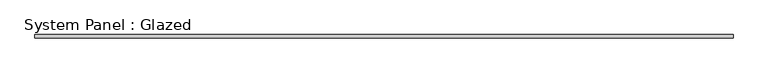
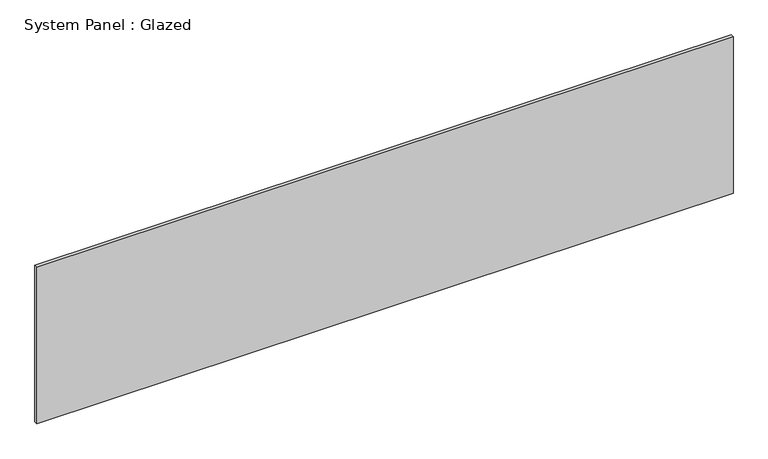
"""IFC4 building model written with IfcOpenShell, lengths in millimetres: plate geometry, System Panel : Glazed."""

from ifc_helpers import new_model, si_unit, origin, origin_with_axes, place, context, project, spatial, polyline, outline, extrude, source, transform, mapped, element, save


def system_panel_glazed_83eff035(model_context):
    return source(origin(), model_context, "Body", "SweptSolid", [
        extrude(outline(polyline([(2565.4, 19.05), (-2565.4, 19.05), (-2565.4, 44.45), (2565.4, 44.45), (2565.4, 19.05)])), origin_with_axes(), (0.0, 0.0, 1.0), 1219.2),
    ])


if __name__ == "__main__":
    model = new_model("IFC4")
    model_context = context("Model", 3, world=origin())
    ifc_project = project(units=[si_unit("LENGTHUNIT", "METRE", prefix="MILLI")], contexts=[model_context])
    site = spatial("IfcSite", under=ifc_project)
    building = spatial("IfcBuilding", under=site)
    placement = place(None, origin())
    system_panel_glazed_shape = system_panel_glazed_83eff035(model_context)
    element("IfcPlate", 1, ObjectType="System Panel : Glazed", at=placement, inside=building, context=model_context, shape_type="MappedRepresentation", body=[
        mapped(system_panel_glazed_shape, transform((0.0, 0.0, 0.0), x_axis=(1.0, 0.0, 0.0), y_axis=(0.0, 1.0, 0.0), z_axis=(0.0, 0.0, 1.0))),
    ])
    save(model, "model.ifc")

# Revit data of these elements
# Type "System Panel : Glazed"
#   Construction Type Id = "GSP4R"
#   Analytic Construction = "1/8 in Pilkington single glazing"
#   Visual Light Transmittance = 0.9
#   Solar Heat Gain Coefficient = 0.86
#   Heat Transfer Coefficient (U) = 1.18115 BTU/(h·ft²·°F)
# Element 1 (IfcPlate, "System Panel : Glazed")
#   Materials on its faces: "Glass"
# Materials
#   "Glass": class "Glass", colour RGB 0 128 192, transparency 0.75, Description = "Soda Lime Glass", Cost = 0
